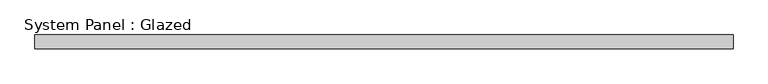
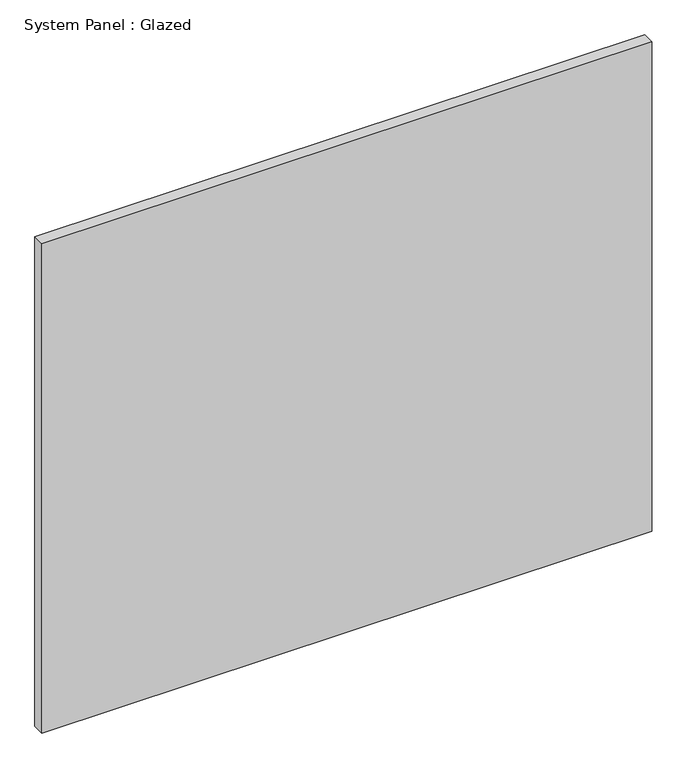
"""IFC4 building model written with IfcOpenShell, lengths in millimetres: plate geometry, System Panel : Glazed."""

from ifc_helpers import new_model, si_unit, origin, origin_with_axes, place, context, project, spatial, polyline, outline, extrude, source, transform, mapped, element, save


def system_panel_glazed_fba3dfff(model_context):
    return source(origin(), model_context, "Body", "SweptSolid", [
        extrude(outline(polyline([(643.9966047, 19.05), (-643.9966047, 19.05), (-643.9966047, 44.45), (643.9966047, 44.45), (643.9966047, 19.05)])), origin_with_axes(), (0.0, 0.0, 1.0), 1092.2),
    ])


if __name__ == "__main__":
    model = new_model("IFC4")
    model_context = context("Model", 3, world=origin())
    ifc_project = project(units=[si_unit("LENGTHUNIT", "METRE", prefix="MILLI")], contexts=[model_context])
    site = spatial("IfcSite", under=ifc_project)
    building = spatial("IfcBuilding", under=site)
    placement = place(None, origin())
    system_panel_glazed_shape = system_panel_glazed_fba3dfff(model_context)
    element("IfcPlate", 1, ObjectType="System Panel : Glazed", at=placement, inside=building, context=model_context, shape_type="MappedRepresentation", body=[
        mapped(system_panel_glazed_shape, transform((0.0, 0.0, 0.0), x_axis=(1.0, 0.0, 0.0), y_axis=(0.0, 1.0, 0.0), z_axis=(0.0, 0.0, 1.0))),
    ])
    save(model, "model.ifc")

# Revit data of these elements
# Type "System Panel : Glazed"
#   Construction Type Id = "GSP4R"
#   Analytic Construction = "1/8 in Pilkington single glazing"
#   Visual Light Transmittance = 0.9
#   Solar Heat Gain Coefficient = 0.86
#   Heat Transfer Coefficient (U) = 1.18115 BTU/(h·ft²·°F)
#   Define Thermal Properties by = 1
# Element 1 (IfcPlate, "System Panel : Glazed")
#   Materials on its faces: "Glass"
# Materials
#   "Glass": class "Glass", colour RGB 0 128 192, transparency 0.75, Description = "Soda Lime Glass", Cost = 0
